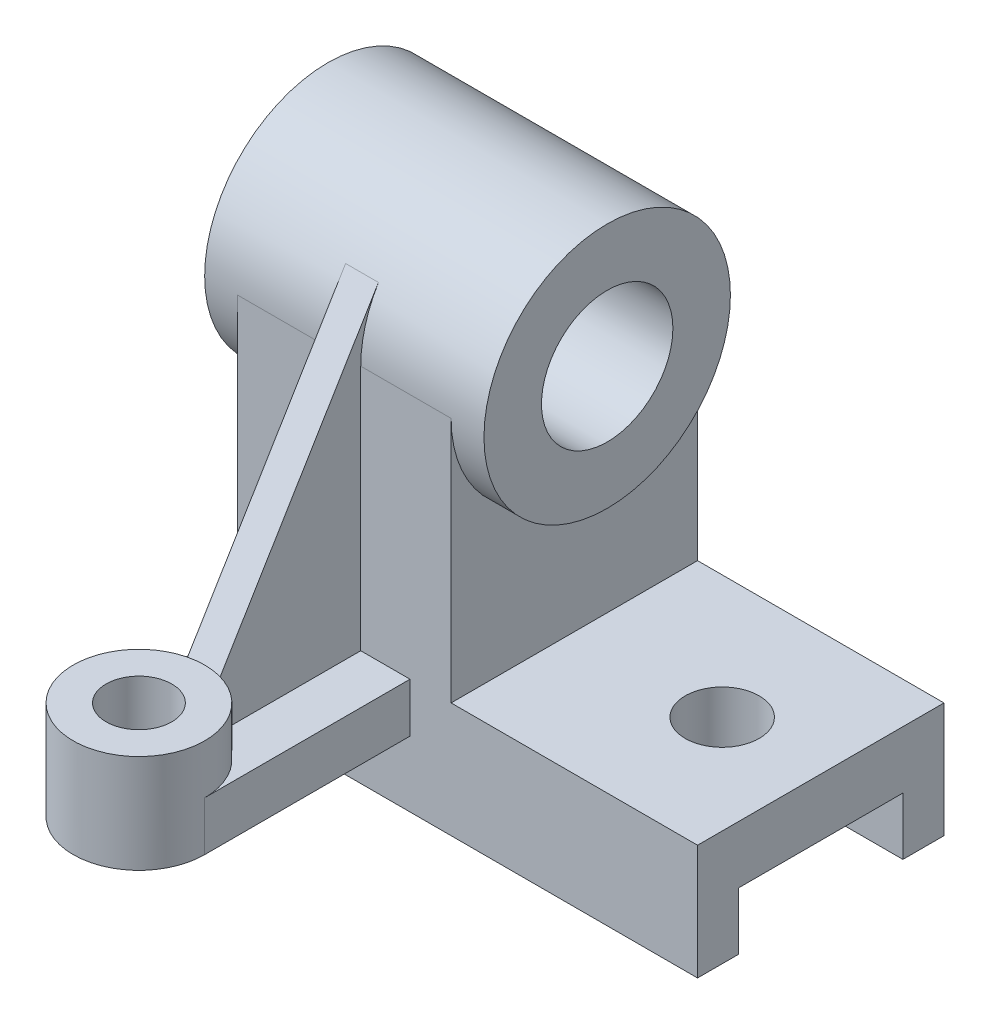
ISO-10303-21;
HEADER;
FILE_DESCRIPTION(('STEP AP214'),'2;1');
FILE_NAME('part.step','',(''),(''),'','','');
FILE_SCHEMA(('AUTOMOTIVE_DESIGN { 1 0 10303 214 1 1 1 1 }'));
ENDSEC;
DATA;
#1=APPLICATION_CONTEXT('core data for automotive mechanical design processes');
#2=APPLICATION_PROTOCOL_DEFINITION('international standard','automotive_design',2000,#1);
#3=PRODUCT_CONTEXT('',#1,'mechanical');
#4=PRODUCT('Part','Part','',(#3));
#5=PRODUCT_RELATED_PRODUCT_CATEGORY('part','',(#4));
#6=PRODUCT_DEFINITION_FORMATION('','',#4);
#7=PRODUCT_DEFINITION_CONTEXT('part definition',#1,'design');
#8=PRODUCT_DEFINITION('design','',#6,#7);
#9=PRODUCT_DEFINITION_SHAPE('','',#8);
#10=(LENGTH_UNIT() NAMED_UNIT(*) SI_UNIT(.MILLI.,.METRE.));
#11=(NAMED_UNIT(*) PLANE_ANGLE_UNIT() SI_UNIT($,.RADIAN.));
#12=(NAMED_UNIT(*) SI_UNIT($,.STERADIAN.) SOLID_ANGLE_UNIT());
#13=UNCERTAINTY_MEASURE_WITH_UNIT(LENGTH_MEASURE(1.E-05),#10,'distance_accuracy_value','');
#14=(GEOMETRIC_REPRESENTATION_CONTEXT(3) GLOBAL_UNCERTAINTY_ASSIGNED_CONTEXT((#13)) GLOBAL_UNIT_ASSIGNED_CONTEXT((#10,
#11,#12)) REPRESENTATION_CONTEXT('',''));
#15=CARTESIAN_POINT('',(0.,0.,0.));
#16=DIRECTION('',(0.,0.,1.));
#17=DIRECTION('',(1.,0.,0.));
#18=AXIS2_PLACEMENT_3D('',#15,#16,#17);
#19=CARTESIAN_POINT('',(0.,-60.,0.));
#20=DIRECTION('',(0.,1.,0.));
#21=DIRECTION('',(0.,0.,1.));
#22=AXIS2_PLACEMENT_3D('',#19,#20,#21);
#23=PLANE('',#22);
#24=CARTESIAN_POINT('',(0.,-60.,80.));
#25=DIRECTION('',(0.,1.,0.));
#26=DIRECTION('',(0.,0.,1.));
#27=AXIS2_PLACEMENT_3D('',#24,#25,#26);
#28=CIRCLE('',#27,16.);
#29=CARTESIAN_POINT('',(-4.,-60.,64.5080666151703));
#30=VERTEX_POINT('',#29);
#31=CARTESIAN_POINT('',(-16.,-60.,80.));
#32=VERTEX_POINT('',#31);
#33=EDGE_CURVE('E195',#30,#32,#28,.T.);
#34=ORIENTED_EDGE('',*,*,#33,.F.);
#35=DIRECTION('',(0.,0.,-1.));
#36=VECTOR('',#35,1.);
#37=CARTESIAN_POINT('',(-4.,-60.,0.));
#38=LINE('',#37,#36);
#39=CARTESIAN_POINT('',(-4.,-60.,30.));
#40=VERTEX_POINT('',#39);
#41=EDGE_CURVE('E191',#30,#40,#38,.T.);
#42=ORIENTED_EDGE('',*,*,#41,.T.);
#43=DIRECTION('',(-1.,0.,0.));
#44=VECTOR('',#43,1.);
#45=CARTESIAN_POINT('',(-16.,-60.,30.));
#46=LINE('',#45,#44);
#47=CARTESIAN_POINT('',(-16.,-60.,30.));
#48=VERTEX_POINT('',#47);
#49=EDGE_CURVE('E172',#40,#48,#46,.T.);
#50=ORIENTED_EDGE('',*,*,#49,.T.);
#51=DIRECTION('',(0.,0.,1.));
#52=VECTOR('',#51,1.);
#53=CARTESIAN_POINT('',(-16.,-60.,30.));
#54=LINE('',#53,#52);
#55=EDGE_CURVE('E227',#48,#32,#54,.T.);
#56=ORIENTED_EDGE('',*,*,#55,.T.);
#57=EDGE_LOOP('',(#34,#42,#50,#56));
#58=FACE_BOUND('',#57,.T.);
#59=ADVANCED_FACE('F41',(#58),#23,.T.);
#60=DIRECTION('',(0.,0.,-1.));
#61=VECTOR('',#60,1.);
#62=CARTESIAN_POINT('',(4.,-60.,0.));
#63=LINE('',#62,#61);
#64=CARTESIAN_POINT('',(4.,-60.,64.5080666151703));
#65=VERTEX_POINT('',#64);
#66=CARTESIAN_POINT('',(4.,-60.,30.));
#67=VERTEX_POINT('',#66);
#68=EDGE_CURVE('E215',#65,#67,#63,.T.);
#69=ORIENTED_EDGE('',*,*,#68,.F.);
#70=CARTESIAN_POINT('',(16.,-60.,80.));
#71=VERTEX_POINT('',#70);
#72=EDGE_CURVE('E234',#71,#65,#28,.T.);
#73=ORIENTED_EDGE('',*,*,#72,.F.);
#74=DIRECTION('',(0.,0.,-1.));
#75=VECTOR('',#74,1.);
#76=CARTESIAN_POINT('',(16.,-60.,30.));
#77=LINE('',#76,#75);
#78=CARTESIAN_POINT('',(16.,-60.,30.));
#79=VERTEX_POINT('',#78);
#80=EDGE_CURVE('E186',#71,#79,#77,.T.);
#81=ORIENTED_EDGE('',*,*,#80,.T.);
#82=EDGE_CURVE('E190',#79,#67,#46,.T.);
#83=ORIENTED_EDGE('',*,*,#82,.T.);
#84=EDGE_LOOP('',(#69,#73,#81,#83));
#85=FACE_BOUND('',#84,.T.);
#86=ADVANCED_FACE('F410',(#85),#23,.T.);
#87=CARTESIAN_POINT('',(0.,-60.,80.));
#88=DIRECTION('',(0.,1.,0.));
#89=DIRECTION('',(0.,0.,1.));
#90=AXIS2_PLACEMENT_3D('',#87,#88,#89);
#91=CYLINDRICAL_SURFACE('',#90,16.);
#92=DIRECTION('',(0.,1.,0.));
#93=VECTOR('',#92,1.);
#94=CARTESIAN_POINT('',(4.,-60.,64.5080666151703));
#95=LINE('',#94,#93);
#96=CARTESIAN_POINT('',(4.,-48.8420392680333,64.5080666151703));
#97=VERTEX_POINT('',#96);
#98=EDGE_CURVE('E60',#97,#65,#95,.F.);
#99=ORIENTED_EDGE('',*,*,#98,.F.);
#100=CARTESIAN_POINT('',(0.,-74.5174445363139,80.));
#101=DIRECTION('',(0.,-0.516619848709566,-0.856214886532175));
#102=DIRECTION('',(0.,0.856214886532175,-0.516619848709566));
#103=AXIS2_PLACEMENT_3D('',#100,#101,#102);
#104=ELLIPSE('',#103,30.9705483441363,16.);
#105=CARTESIAN_POINT('',(0.,-48.,64.));
#106=VERTEX_POINT('',#105);
#107=EDGE_CURVE('E219',#106,#97,#104,.T.);
#108=ORIENTED_EDGE('',*,*,#107,.F.);
#109=CARTESIAN_POINT('',(0.,-48.,80.));
#110=DIRECTION('',(0.,1.,0.));
#111=DIRECTION('',(0.,0.,1.));
#112=AXIS2_PLACEMENT_3D('',#109,#110,#111);
#113=CIRCLE('',#112,16.);
#114=EDGE_CURVE('E230',#106,#106,#113,.T.);
#115=ORIENTED_EDGE('',*,*,#114,.F.);
#116=CARTESIAN_POINT('',(-4.,-48.8420392680333,64.5080666151703));
#117=VERTEX_POINT('',#116);
#118=EDGE_CURVE('E64',#117,#106,#104,.T.);
#119=ORIENTED_EDGE('',*,*,#118,.F.);
#120=DIRECTION('',(0.,1.,0.));
#121=VECTOR('',#120,1.);
#122=CARTESIAN_POINT('',(-4.,-60.,64.5080666151703));
#123=LINE('',#122,#121);
#124=EDGE_CURVE('E192',#117,#30,#123,.F.);
#125=ORIENTED_EDGE('',*,*,#124,.T.);
#126=ORIENTED_EDGE('',*,*,#33,.T.);
#127=DIRECTION('',(0.,1.,0.));
#128=VECTOR('',#127,1.);
#129=CARTESIAN_POINT('',(-16.,-72.,80.));
#130=LINE('',#129,#128);
#131=CARTESIAN_POINT('',(-16.,-72.,80.));
#132=VERTEX_POINT('',#131);
#133=EDGE_CURVE('E49',#132,#32,#130,.T.);
#134=ORIENTED_EDGE('',*,*,#133,.F.);
#135=CARTESIAN_POINT('',(0.,-72.,80.));
#136=DIRECTION('',(0.,1.,0.));
#137=DIRECTION('',(0.,0.,1.));
#138=AXIS2_PLACEMENT_3D('',#135,#136,#137);
#139=CIRCLE('',#138,16.);
#140=CARTESIAN_POINT('',(16.,-72.,80.));
#141=VERTEX_POINT('',#140);
#142=EDGE_CURVE('E11',#141,#132,#139,.F.);
#143=ORIENTED_EDGE('',*,*,#142,.F.);
#144=DIRECTION('',(0.,1.,0.));
#145=VECTOR('',#144,1.);
#146=CARTESIAN_POINT('',(16.,-72.,80.));
#147=LINE('',#146,#145);
#148=EDGE_CURVE('E333',#71,#141,#147,.F.);
#149=ORIENTED_EDGE('',*,*,#148,.F.);
#150=ORIENTED_EDGE('',*,*,#72,.T.);
#151=EDGE_LOOP('',(#99,#108,#115,#119,#125,#126,#134,#143,#149,#150));
#152=FACE_BOUND('',#151,.T.);
#153=ADVANCED_FACE('F42',(#152),#91,.T.);
#154=CARTESIAN_POINT('',(86.,-88.,30.));
#155=DIRECTION('',(0.,1.,0.));
#156=DIRECTION('',(-1.,0.,0.));
#157=AXIS2_PLACEMENT_3D('',#154,#155,#156);
#158=PLANE('',#157);
#159=DIRECTION('',(0.,0.,-1.));
#160=VECTOR('',#159,1.);
#161=CARTESIAN_POINT('',(86.,-88.,30.));
#162=LINE('',#161,#160);
#163=CARTESIAN_POINT('',(86.,-88.,-20.));
#164=VERTEX_POINT('',#163);
#165=CARTESIAN_POINT('',(86.,-88.,-30.));
#166=VERTEX_POINT('',#165);
#167=EDGE_CURVE('E303',#164,#166,#162,.T.);
#168=ORIENTED_EDGE('',*,*,#167,.F.);
#169=DIRECTION('',(1.,0.,0.));
#170=VECTOR('',#169,1.);
#171=CARTESIAN_POINT('',(-34.,-88.,-20.));
#172=LINE('',#171,#170);
#173=CARTESIAN_POINT('',(-26.,-88.,-20.));
#174=VERTEX_POINT('',#173);
#175=EDGE_CURVE('E266',#174,#164,#172,.T.);
#176=ORIENTED_EDGE('',*,*,#175,.F.);
#177=DIRECTION('',(0.,0.,-1.));
#178=VECTOR('',#177,1.);
#179=CARTESIAN_POINT('',(-26.,-88.,30.));
#180=LINE('',#179,#178);
#181=CARTESIAN_POINT('',(-26.,-88.,-30.));
#182=VERTEX_POINT('',#181);
#183=EDGE_CURVE('E306',#174,#182,#180,.T.);
#184=ORIENTED_EDGE('',*,*,#183,.T.);
#185=DIRECTION('',(1.,0.,0.));
#186=VECTOR('',#185,1.);
#187=CARTESIAN_POINT('',(86.,-88.,-30.));
#188=LINE('',#187,#186);
#189=EDGE_CURVE('E292',#182,#166,#188,.T.);
#190=ORIENTED_EDGE('',*,*,#189,.T.);
#191=EDGE_LOOP('',(#168,#176,#184,#190));
#192=FACE_BOUND('',#191,.T.);
#193=ADVANCED_FACE('F401',(#192),#158,.F.);
#194=CARTESIAN_POINT('',(86.,-60.,30.));
#195=DIRECTION('',(-1.,0.,0.));
#196=DIRECTION('',(0.,0.,1.));
#197=AXIS2_PLACEMENT_3D('',#194,#195,#196);
#198=PLANE('',#197);
#199=DIRECTION('',(0.,-1.,0.));
#200=VECTOR('',#199,1.);
#201=CARTESIAN_POINT('',(86.,-88.,20.));
#202=LINE('',#201,#200);
#203=CARTESIAN_POINT('',(86.,-74.,20.));
#204=VERTEX_POINT('',#203);
#205=CARTESIAN_POINT('',(86.,-88.,20.));
#206=VERTEX_POINT('',#205);
#207=EDGE_CURVE('E253',#204,#206,#202,.T.);
#208=ORIENTED_EDGE('',*,*,#207,.F.);
#209=DIRECTION('',(0.,0.,1.));
#210=VECTOR('',#209,1.);
#211=CARTESIAN_POINT('',(86.,-74.,20.));
#212=LINE('',#211,#210);
#213=CARTESIAN_POINT('',(86.,-74.,-20.));
#214=VERTEX_POINT('',#213);
#215=EDGE_CURVE('E260',#214,#204,#212,.T.);
#216=ORIENTED_EDGE('',*,*,#215,.F.);
#217=DIRECTION('',(0.,1.,0.));
#218=VECTOR('',#217,1.);
#219=CARTESIAN_POINT('',(86.,-88.,-20.));
#220=LINE('',#219,#218);
#221=EDGE_CURVE('E255',#164,#214,#220,.T.);
#222=ORIENTED_EDGE('',*,*,#221,.F.);
#223=ORIENTED_EDGE('',*,*,#167,.T.);
#224=DIRECTION('',(0.,1.,0.));
#225=VECTOR('',#224,1.);
#226=CARTESIAN_POINT('',(86.,-60.,-30.));
#227=LINE('',#226,#225);
#228=CARTESIAN_POINT('',(86.,-60.,-30.));
#229=VERTEX_POINT('',#228);
#230=EDGE_CURVE('E291',#166,#229,#227,.T.);
#231=ORIENTED_EDGE('',*,*,#230,.T.);
#232=DIRECTION('',(0.,0.,-1.));
#233=VECTOR('',#232,1.);
#234=CARTESIAN_POINT('',(86.,-60.,30.));
#235=LINE('',#234,#233);
#236=CARTESIAN_POINT('',(86.,-60.,30.));
#237=VERTEX_POINT('',#236);
#238=EDGE_CURVE('E304',#237,#229,#235,.T.);
#239=ORIENTED_EDGE('',*,*,#238,.F.);
#240=DIRECTION('',(0.,1.,0.));
#241=VECTOR('',#240,1.);
#242=CARTESIAN_POINT('',(86.,-60.,30.));
#243=LINE('',#242,#241);
#244=CARTESIAN_POINT('',(86.,-88.,30.));
#245=VERTEX_POINT('',#244);
#246=EDGE_CURVE('E276',#245,#237,#243,.T.);
#247=ORIENTED_EDGE('',*,*,#246,.F.);
#248=EDGE_CURVE('E302',#245,#206,#162,.T.);
#249=ORIENTED_EDGE('',*,*,#248,.T.);
#250=EDGE_LOOP('',(#208,#216,#222,#223,#231,#239,#247,#249));
#251=FACE_BOUND('',#250,.T.);
#252=ADVANCED_FACE('F390',(#251),#198,.F.);
#253=CARTESIAN_POINT('',(34.,0.,0.));
#254=DIRECTION('',(-1.,0.,0.));
#255=DIRECTION('',(0.,0.,1.));
#256=AXIS2_PLACEMENT_3D('',#253,#254,#255);
#257=CYLINDRICAL_SURFACE('',#256,30.);
#258=CARTESIAN_POINT('',(34.,0.,0.));
#259=DIRECTION('',(1.,0.,0.));
#260=DIRECTION('',(0.,0.,-1.));
#261=AXIS2_PLACEMENT_3D('',#258,#259,#260);
#262=CIRCLE('',#261,30.);
#263=CARTESIAN_POINT('',(34.,0.,-30.));
#264=VERTEX_POINT('',#263);
#265=EDGE_CURVE('E322',#264,#264,#262,.T.);
#266=ORIENTED_EDGE('',*,*,#265,.F.);
#267=EDGE_LOOP('',(#266));
#268=FACE_BOUND('',#267,.T.);
#269=DIRECTION('',(-1.,0.,0.));
#270=VECTOR('',#269,1.);
#271=CARTESIAN_POINT('',(-26.,0.,-30.));
#272=LINE('',#271,#270);
#273=CARTESIAN_POINT('',(26.,0.,-30.));
#274=VERTEX_POINT('',#273);
#275=CARTESIAN_POINT('',(-26.,0.,-30.));
#276=VERTEX_POINT('',#275);
#277=EDGE_CURVE('E271',#274,#276,#272,.T.);
#278=ORIENTED_EDGE('',*,*,#277,.T.);
#279=CARTESIAN_POINT('',(-26.,0.,0.));
#280=DIRECTION('',(1.,0.,0.));
#281=DIRECTION('',(0.,1.,0.));
#282=AXIS2_PLACEMENT_3D('',#279,#280,#281);
#283=CIRCLE('',#282,30.);
#284=CARTESIAN_POINT('',(-26.,0.,30.));
#285=VERTEX_POINT('',#284);
#286=EDGE_CURVE('E314',#285,#276,#283,.T.);
#287=ORIENTED_EDGE('',*,*,#286,.F.);
#288=DIRECTION('',(-1.,0.,0.));
#289=VECTOR('',#288,1.);
#290=CARTESIAN_POINT('',(-26.,0.,30.));
#291=LINE('',#290,#289);
#292=CARTESIAN_POINT('',(-4.,0.,30.));
#293=VERTEX_POINT('',#292);
#294=EDGE_CURVE('E274',#293,#285,#291,.T.);
#295=ORIENTED_EDGE('',*,*,#294,.F.);
#296=CARTESIAN_POINT('',(-4.,0.,0.));
#297=DIRECTION('',(1.,0.,0.));
#298=DIRECTION('',(0.,0.,-1.));
#299=AXIS2_PLACEMENT_3D('',#296,#297,#298);
#300=CIRCLE('',#299,30.);
#301=CARTESIAN_POINT('',(-4.,15.498595461287,25.6864465959653));
#302=VERTEX_POINT('',#301);
#303=EDGE_CURVE('E199',#302,#293,#300,.T.);
#304=ORIENTED_EDGE('',*,*,#303,.F.);
#305=DIRECTION('',(-1.,0.,0.));
#306=VECTOR('',#305,1.);
#307=CARTESIAN_POINT('',(34.,15.498595461287,25.6864465959652));
#308=LINE('',#307,#306);
#309=CARTESIAN_POINT('',(4.,15.498595461287,25.6864465959653));
#310=VERTEX_POINT('',#309);
#311=EDGE_CURVE('E220',#302,#310,#308,.F.);
#312=ORIENTED_EDGE('',*,*,#311,.T.);
#313=CARTESIAN_POINT('',(4.,0.,0.));
#314=DIRECTION('',(1.,0.,0.));
#315=DIRECTION('',(0.,0.,-1.));
#316=AXIS2_PLACEMENT_3D('',#313,#314,#315);
#317=CIRCLE('',#316,30.);
#318=CARTESIAN_POINT('',(4.,0.,30.));
#319=VERTEX_POINT('',#318);
#320=EDGE_CURVE('E207',#310,#319,#317,.T.);
#321=ORIENTED_EDGE('',*,*,#320,.T.);
#322=CARTESIAN_POINT('',(26.,0.,30.));
#323=VERTEX_POINT('',#322);
#324=EDGE_CURVE('E275',#323,#319,#291,.T.);
#325=ORIENTED_EDGE('',*,*,#324,.F.);
#326=CARTESIAN_POINT('',(26.,0.,0.));
#327=DIRECTION('',(-1.,0.,0.));
#328=DIRECTION('',(0.,-1.,0.));
#329=AXIS2_PLACEMENT_3D('',#326,#327,#328);
#330=CIRCLE('',#329,30.);
#331=EDGE_CURVE('E315',#274,#323,#330,.T.);
#332=ORIENTED_EDGE('',*,*,#331,.F.);
#333=EDGE_LOOP('',(#278,#287,#295,#304,#312,#321,#325,#332));
#334=FACE_BOUND('',#333,.T.);
#335=CARTESIAN_POINT('',(-34.,0.,0.));
#336=DIRECTION('',(1.,0.,0.));
#337=DIRECTION('',(0.,0.,-1.));
#338=AXIS2_PLACEMENT_3D('',#335,#336,#337);
#339=CIRCLE('',#338,30.);
#340=CARTESIAN_POINT('',(-34.,0.,-30.));
#341=VERTEX_POINT('',#340);
#342=EDGE_CURVE('E321',#341,#341,#339,.T.);
#343=ORIENTED_EDGE('',*,*,#342,.T.);
#344=EDGE_LOOP('',(#343));
#345=FACE_BOUND('',#344,.T.);
#346=ADVANCED_FACE('F356',(#268,#334,#345),#257,.T.);
#347=CARTESIAN_POINT('',(34.,0.,0.));
#348=DIRECTION('',(-1.,0.,0.));
#349=DIRECTION('',(0.,0.,1.));
#350=AXIS2_PLACEMENT_3D('',#347,#348,#349);
#351=CYLINDRICAL_SURFACE('',#350,16.);
#352=CARTESIAN_POINT('',(34.,0.,0.));
#353=DIRECTION('',(1.,0.,0.));
#354=DIRECTION('',(0.,0.,-1.));
#355=AXIS2_PLACEMENT_3D('',#352,#353,#354);
#356=CIRCLE('',#355,16.);
#357=CARTESIAN_POINT('',(34.,0.,-16.));
#358=VERTEX_POINT('',#357);
#359=EDGE_CURVE('E318',#358,#358,#356,.T.);
#360=ORIENTED_EDGE('',*,*,#359,.T.);
#361=EDGE_LOOP('',(#360));
#362=FACE_BOUND('',#361,.T.);
#363=CARTESIAN_POINT('',(-34.,0.,0.));
#364=DIRECTION('',(1.,0.,0.));
#365=DIRECTION('',(0.,0.,-1.));
#366=AXIS2_PLACEMENT_3D('',#363,#364,#365);
#367=CIRCLE('',#366,16.);
#368=CARTESIAN_POINT('',(-34.,0.,-16.));
#369=VERTEX_POINT('',#368);
#370=EDGE_CURVE('E320',#369,#369,#367,.T.);
#371=ORIENTED_EDGE('',*,*,#370,.F.);
#372=EDGE_LOOP('',(#371));
#373=FACE_BOUND('',#372,.T.);
#374=ADVANCED_FACE('F599',(#362,#373),#351,.F.);
#375=CARTESIAN_POINT('',(34.,0.,0.));
#376=DIRECTION('',(1.,0.,0.));
#377=DIRECTION('',(0.,0.,-1.));
#378=AXIS2_PLACEMENT_3D('',#375,#376,#377);
#379=PLANE('',#378);
#380=ORIENTED_EDGE('',*,*,#265,.T.);
#381=EDGE_LOOP('',(#380));
#382=FACE_BOUND('',#381,.T.);
#383=ORIENTED_EDGE('',*,*,#359,.F.);
#384=EDGE_LOOP('',(#383));
#385=FACE_BOUND('',#384,.T.);
#386=ADVANCED_FACE('F606',(#382,#385),#379,.T.);
#387=CARTESIAN_POINT('',(-34.,0.,0.));
#388=DIRECTION('',(1.,0.,0.));
#389=DIRECTION('',(0.,0.,-1.));
#390=AXIS2_PLACEMENT_3D('',#387,#388,#389);
#391=PLANE('',#390);
#392=ORIENTED_EDGE('',*,*,#342,.F.);
#393=EDGE_LOOP('',(#392));
#394=FACE_BOUND('',#393,.T.);
#395=ORIENTED_EDGE('',*,*,#370,.T.);
#396=EDGE_LOOP('',(#395));
#397=FACE_BOUND('',#396,.T.);
#398=ADVANCED_FACE('F593',(#394,#397),#391,.F.);
#399=CARTESIAN_POINT('',(-26.,-88.,30.));
#400=DIRECTION('',(1.,0.,0.));
#401=DIRECTION('',(0.,1.,0.));
#402=AXIS2_PLACEMENT_3D('',#399,#400,#401);
#403=PLANE('',#402);
#404=DIRECTION('',(0.,0.,1.));
#405=VECTOR('',#404,1.);
#406=CARTESIAN_POINT('',(-26.,-74.,30.));
#407=LINE('',#406,#405);
#408=CARTESIAN_POINT('',(-26.,-74.,-20.));
#409=VERTEX_POINT('',#408);
#410=CARTESIAN_POINT('',(-26.,-74.,20.));
#411=VERTEX_POINT('',#410);
#412=EDGE_CURVE('E263',#409,#411,#407,.T.);
#413=ORIENTED_EDGE('',*,*,#412,.T.);
#414=DIRECTION('',(0.,-1.,0.));
#415=VECTOR('',#414,1.);
#416=CARTESIAN_POINT('',(-26.,-88.,20.));
#417=LINE('',#416,#415);
#418=CARTESIAN_POINT('',(-26.,-88.,20.));
#419=VERTEX_POINT('',#418);
#420=EDGE_CURVE('E335',#411,#419,#417,.T.);
#421=ORIENTED_EDGE('',*,*,#420,.T.);
#422=CARTESIAN_POINT('',(-26.,-88.,30.));
#423=VERTEX_POINT('',#422);
#424=EDGE_CURVE('E310',#423,#419,#180,.T.);
#425=ORIENTED_EDGE('',*,*,#424,.F.);
#426=DIRECTION('',(0.,-1.,0.));
#427=VECTOR('',#426,1.);
#428=CARTESIAN_POINT('',(-26.,-88.,30.));
#429=LINE('',#428,#427);
#430=EDGE_CURVE('E273',#285,#423,#429,.T.);
#431=ORIENTED_EDGE('',*,*,#430,.F.);
#432=ORIENTED_EDGE('',*,*,#286,.T.);
#433=DIRECTION('',(0.,-1.,0.));
#434=VECTOR('',#433,1.);
#435=CARTESIAN_POINT('',(-26.,-88.,-30.));
#436=LINE('',#435,#434);
#437=EDGE_CURVE('E290',#276,#182,#436,.T.);
#438=ORIENTED_EDGE('',*,*,#437,.T.);
#439=ORIENTED_EDGE('',*,*,#183,.F.);
#440=DIRECTION('',(0.,1.,0.));
#441=VECTOR('',#440,1.);
#442=CARTESIAN_POINT('',(-26.,-88.,-20.));
#443=LINE('',#442,#441);
#444=EDGE_CURVE('E330',#174,#409,#443,.T.);
#445=ORIENTED_EDGE('',*,*,#444,.T.);
#446=EDGE_LOOP('',(#413,#421,#425,#431,#432,#438,#439,#445));
#447=FACE_BOUND('',#446,.T.);
#448=ADVANCED_FACE('F380',(#447),#403,.F.);
#449=ORIENTED_EDGE('',*,*,#248,.F.);
#450=DIRECTION('',(1.,0.,0.));
#451=VECTOR('',#450,1.);
#452=CARTESIAN_POINT('',(86.,-88.,30.));
#453=LINE('',#452,#451);
#454=EDGE_CURVE('E280',#423,#245,#453,.T.);
#455=ORIENTED_EDGE('',*,*,#454,.F.);
#456=ORIENTED_EDGE('',*,*,#424,.T.);
#457=DIRECTION('',(1.,0.,0.));
#458=VECTOR('',#457,1.);
#459=CARTESIAN_POINT('',(-34.,-88.,20.));
#460=LINE('',#459,#458);
#461=EDGE_CURVE('E257',#419,#206,#460,.T.);
#462=ORIENTED_EDGE('',*,*,#461,.T.);
#463=EDGE_LOOP('',(#449,#455,#456,#462));
#464=FACE_BOUND('',#463,.T.);
#465=ADVANCED_FACE('F383',(#464),#158,.F.);
#466=CARTESIAN_POINT('',(26.,-60.,30.));
#467=DIRECTION('',(0.,-1.,0.));
#468=DIRECTION('',(0.,0.,-1.));
#469=AXIS2_PLACEMENT_3D('',#466,#467,#468);
#470=PLANE('',#469);
#471=CARTESIAN_POINT('',(62.,-60.,0.));
#472=DIRECTION('',(0.,1.,0.));
#473=DIRECTION('',(0.,0.,1.));
#474=AXIS2_PLACEMENT_3D('',#471,#472,#473);
#475=CIRCLE('',#474,9.);
#476=CARTESIAN_POINT('',(62.,-60.,9.));
#477=VERTEX_POINT('',#476);
#478=EDGE_CURVE('E242',#477,#477,#475,.T.);
#479=ORIENTED_EDGE('',*,*,#478,.F.);
#480=EDGE_LOOP('',(#479));
#481=FACE_BOUND('',#480,.T.);
#482=DIRECTION('',(-1.,0.,0.));
#483=VECTOR('',#482,1.);
#484=CARTESIAN_POINT('',(26.,-60.,-30.));
#485=LINE('',#484,#483);
#486=CARTESIAN_POINT('',(26.,-60.,-30.));
#487=VERTEX_POINT('',#486);
#488=EDGE_CURVE('E293',#229,#487,#485,.T.);
#489=ORIENTED_EDGE('',*,*,#488,.T.);
#490=DIRECTION('',(0.,0.,-1.));
#491=VECTOR('',#490,1.);
#492=CARTESIAN_POINT('',(26.,-60.,30.));
#493=LINE('',#492,#491);
#494=CARTESIAN_POINT('',(26.,-60.,30.));
#495=VERTEX_POINT('',#494);
#496=EDGE_CURVE('E289',#495,#487,#493,.T.);
#497=ORIENTED_EDGE('',*,*,#496,.F.);
#498=DIRECTION('',(-1.,0.,0.));
#499=VECTOR('',#498,1.);
#500=CARTESIAN_POINT('',(26.,-60.,30.));
#501=LINE('',#500,#499);
#502=EDGE_CURVE('E283',#237,#495,#501,.T.);
#503=ORIENTED_EDGE('',*,*,#502,.F.);
#504=ORIENTED_EDGE('',*,*,#238,.T.);
#505=EDGE_LOOP('',(#489,#497,#503,#504));
#506=FACE_BOUND('',#505,.T.);
#507=ADVANCED_FACE('F393',(#481,#506),#470,.F.);
#508=CARTESIAN_POINT('',(26.,0.,30.));
#509=DIRECTION('',(-1.,0.,0.));
#510=DIRECTION('',(0.,-1.,0.));
#511=AXIS2_PLACEMENT_3D('',#508,#509,#510);
#512=PLANE('',#511);
#513=DIRECTION('',(0.,1.,0.));
#514=VECTOR('',#513,1.);
#515=CARTESIAN_POINT('',(26.,0.,-30.));
#516=LINE('',#515,#514);
#517=EDGE_CURVE('E300',#487,#274,#516,.T.);
#518=ORIENTED_EDGE('',*,*,#517,.T.);
#519=ORIENTED_EDGE('',*,*,#331,.T.);
#520=DIRECTION('',(0.,1.,0.));
#521=VECTOR('',#520,1.);
#522=CARTESIAN_POINT('',(26.,0.,30.));
#523=LINE('',#522,#521);
#524=EDGE_CURVE('E281',#495,#323,#523,.T.);
#525=ORIENTED_EDGE('',*,*,#524,.F.);
#526=ORIENTED_EDGE('',*,*,#496,.T.);
#527=EDGE_LOOP('',(#518,#519,#525,#526));
#528=FACE_BOUND('',#527,.T.);
#529=ADVANCED_FACE('F364',(#528),#512,.F.);
#530=CARTESIAN_POINT('',(0.,0.,30.));
#531=DIRECTION('',(0.,0.,-1.));
#532=DIRECTION('',(-1.,0.,0.));
#533=AXIS2_PLACEMENT_3D('',#530,#531,#532);
#534=PLANE('',#533);
#535=ORIENTED_EDGE('',*,*,#324,.T.);
#536=DIRECTION('',(0.,-1.,0.));
#537=VECTOR('',#536,1.);
#538=CARTESIAN_POINT('',(4.,0.,30.));
#539=LINE('',#538,#537);
#540=EDGE_CURVE('E209',#319,#67,#539,.T.);
#541=ORIENTED_EDGE('',*,*,#540,.T.);
#542=ORIENTED_EDGE('',*,*,#82,.F.);
#543=DIRECTION('',(0.,1.,0.));
#544=VECTOR('',#543,1.);
#545=CARTESIAN_POINT('',(16.,-72.,30.));
#546=LINE('',#545,#544);
#547=CARTESIAN_POINT('',(16.,-72.,30.));
#548=VERTEX_POINT('',#547);
#549=EDGE_CURVE('E238',#548,#79,#546,.T.);
#550=ORIENTED_EDGE('',*,*,#549,.F.);
#551=DIRECTION('',(-1.,0.,0.));
#552=VECTOR('',#551,1.);
#553=CARTESIAN_POINT('',(-16.,-72.,30.));
#554=LINE('',#553,#552);
#555=CARTESIAN_POINT('',(-16.,-72.,30.));
#556=VERTEX_POINT('',#555);
#557=EDGE_CURVE('E236',#548,#556,#554,.T.);
#558=ORIENTED_EDGE('',*,*,#557,.T.);
#559=DIRECTION('',(0.,1.,0.));
#560=VECTOR('',#559,1.);
#561=CARTESIAN_POINT('',(-16.,-72.,30.));
#562=LINE('',#561,#560);
#563=EDGE_CURVE('E181',#556,#48,#562,.T.);
#564=ORIENTED_EDGE('',*,*,#563,.T.);
#565=ORIENTED_EDGE('',*,*,#49,.F.);
#566=DIRECTION('',(0.,-1.,0.));
#567=VECTOR('',#566,1.);
#568=CARTESIAN_POINT('',(-4.,0.,30.));
#569=LINE('',#568,#567);
#570=EDGE_CURVE('E177',#293,#40,#569,.T.);
#571=ORIENTED_EDGE('',*,*,#570,.F.);
#572=ORIENTED_EDGE('',*,*,#294,.T.);
#573=ORIENTED_EDGE('',*,*,#430,.T.);
#574=ORIENTED_EDGE('',*,*,#454,.T.);
#575=ORIENTED_EDGE('',*,*,#246,.T.);
#576=ORIENTED_EDGE('',*,*,#502,.T.);
#577=ORIENTED_EDGE('',*,*,#524,.T.);
#578=EDGE_LOOP('',(#535,#541,#542,#550,#558,#564,#565,#571,#572,#573,#574,#575,#576,#577));
#579=FACE_BOUND('',#578,.T.);
#580=ADVANCED_FACE('F180',(#579),#534,.F.);
#581=CARTESIAN_POINT('',(0.,0.,-30.));
#582=DIRECTION('',(0.,0.,-1.));
#583=DIRECTION('',(-1.,0.,0.));
#584=AXIS2_PLACEMENT_3D('',#581,#582,#583);
#585=PLANE('',#584);
#586=ORIENTED_EDGE('',*,*,#230,.F.);
#587=ORIENTED_EDGE('',*,*,#189,.F.);
#588=ORIENTED_EDGE('',*,*,#437,.F.);
#589=ORIENTED_EDGE('',*,*,#277,.F.);
#590=ORIENTED_EDGE('',*,*,#517,.F.);
#591=ORIENTED_EDGE('',*,*,#488,.F.);
#592=EDGE_LOOP('',(#586,#587,#588,#589,#590,#591));
#593=FACE_BOUND('',#592,.T.);
#594=ADVANCED_FACE('F373',(#593),#585,.T.);
#595=CARTESIAN_POINT('',(-34.,-88.,20.));
#596=DIRECTION('',(0.,0.,1.));
#597=DIRECTION('',(1.,0.,0.));
#598=AXIS2_PLACEMENT_3D('',#595,#596,#597);
#599=PLANE('',#598);
#600=ORIENTED_EDGE('',*,*,#207,.T.);
#601=ORIENTED_EDGE('',*,*,#461,.F.);
#602=ORIENTED_EDGE('',*,*,#420,.F.);
#603=DIRECTION('',(1.,0.,0.));
#604=VECTOR('',#603,1.);
#605=CARTESIAN_POINT('',(-34.,-74.,20.));
#606=LINE('',#605,#604);
#607=EDGE_CURVE('E261',#411,#204,#606,.T.);
#608=ORIENTED_EDGE('',*,*,#607,.T.);
#609=EDGE_LOOP('',(#600,#601,#602,#608));
#610=FACE_BOUND('',#609,.T.);
#611=ADVANCED_FACE('F433',(#610),#599,.F.);
#612=CARTESIAN_POINT('',(-34.,-88.,-20.));
#613=DIRECTION('',(0.,0.,-1.));
#614=DIRECTION('',(-1.,0.,0.));
#615=AXIS2_PLACEMENT_3D('',#612,#613,#614);
#616=PLANE('',#615);
#617=ORIENTED_EDGE('',*,*,#221,.T.);
#618=DIRECTION('',(1.,0.,0.));
#619=VECTOR('',#618,1.);
#620=CARTESIAN_POINT('',(-34.,-74.,-20.));
#621=LINE('',#620,#619);
#622=EDGE_CURVE('E262',#409,#214,#621,.T.);
#623=ORIENTED_EDGE('',*,*,#622,.F.);
#624=ORIENTED_EDGE('',*,*,#444,.F.);
#625=ORIENTED_EDGE('',*,*,#175,.T.);
#626=EDGE_LOOP('',(#617,#623,#624,#625));
#627=FACE_BOUND('',#626,.T.);
#628=ADVANCED_FACE('F427',(#627),#616,.F.);
#629=CARTESIAN_POINT('',(-34.,-74.,20.));
#630=DIRECTION('',(0.,1.,0.));
#631=DIRECTION('',(0.,0.,1.));
#632=AXIS2_PLACEMENT_3D('',#629,#630,#631);
#633=PLANE('',#632);
#634=CARTESIAN_POINT('',(62.,-74.,0.));
#635=DIRECTION('',(0.,1.,0.));
#636=DIRECTION('',(0.,0.,1.));
#637=AXIS2_PLACEMENT_3D('',#634,#635,#636);
#638=CIRCLE('',#637,9.);
#639=CARTESIAN_POINT('',(62.,-74.,9.));
#640=VERTEX_POINT('',#639);
#641=EDGE_CURVE('E247',#640,#640,#638,.T.);
#642=ORIENTED_EDGE('',*,*,#641,.T.);
#643=EDGE_LOOP('',(#642));
#644=FACE_BOUND('',#643,.T.);
#645=ORIENTED_EDGE('',*,*,#215,.T.);
#646=ORIENTED_EDGE('',*,*,#607,.F.);
#647=ORIENTED_EDGE('',*,*,#412,.F.);
#648=ORIENTED_EDGE('',*,*,#622,.T.);
#649=EDGE_LOOP('',(#645,#646,#647,#648));
#650=FACE_BOUND('',#649,.T.);
#651=ADVANCED_FACE('F422',(#644,#650),#633,.F.);
#652=CARTESIAN_POINT('',(62.,-88.,0.));
#653=DIRECTION('',(0.,1.,0.));
#654=DIRECTION('',(0.,0.,1.));
#655=AXIS2_PLACEMENT_3D('',#652,#653,#654);
#656=CYLINDRICAL_SURFACE('',#655,9.);
#657=ORIENTED_EDGE('',*,*,#478,.T.);
#658=EDGE_LOOP('',(#657));
#659=FACE_BOUND('',#658,.T.);
#660=ORIENTED_EDGE('',*,*,#641,.F.);
#661=EDGE_LOOP('',(#660));
#662=FACE_BOUND('',#661,.T.);
#663=ADVANCED_FACE('F421',(#659,#662),#656,.F.);
#664=CARTESIAN_POINT('',(-16.,-72.,30.));
#665=DIRECTION('',(-1.,0.,0.));
#666=DIRECTION('',(0.,0.,1.));
#667=AXIS2_PLACEMENT_3D('',#664,#665,#666);
#668=PLANE('',#667);
#669=DIRECTION('',(0.,0.,1.));
#670=VECTOR('',#669,1.);
#671=CARTESIAN_POINT('',(-16.,-72.,30.));
#672=LINE('',#671,#670);
#673=EDGE_CURVE('E235',#556,#132,#672,.T.);
#674=ORIENTED_EDGE('',*,*,#673,.T.);
#675=ORIENTED_EDGE('',*,*,#133,.T.);
#676=ORIENTED_EDGE('',*,*,#55,.F.);
#677=ORIENTED_EDGE('',*,*,#563,.F.);
#678=EDGE_LOOP('',(#674,#675,#676,#677));
#679=FACE_BOUND('',#678,.T.);
#680=ADVANCED_FACE('F341',(#679),#668,.T.);
#681=CARTESIAN_POINT('',(16.,-72.,30.));
#682=DIRECTION('',(1.,0.,0.));
#683=DIRECTION('',(0.,0.,-1.));
#684=AXIS2_PLACEMENT_3D('',#681,#682,#683);
#685=PLANE('',#684);
#686=ORIENTED_EDGE('',*,*,#80,.F.);
#687=ORIENTED_EDGE('',*,*,#148,.T.);
#688=DIRECTION('',(0.,0.,-1.));
#689=VECTOR('',#688,1.);
#690=CARTESIAN_POINT('',(16.,-72.,30.));
#691=LINE('',#690,#689);
#692=EDGE_CURVE('E237',#141,#548,#691,.T.);
#693=ORIENTED_EDGE('',*,*,#692,.T.);
#694=ORIENTED_EDGE('',*,*,#549,.T.);
#695=EDGE_LOOP('',(#686,#687,#693,#694));
#696=FACE_BOUND('',#695,.T.);
#697=ADVANCED_FACE('F416',(#696),#685,.T.);
#698=CARTESIAN_POINT('',(0.,-72.,0.));
#699=DIRECTION('',(0.,1.,0.));
#700=DIRECTION('',(0.,0.,1.));
#701=AXIS2_PLACEMENT_3D('',#698,#699,#700);
#702=PLANE('',#701);
#703=ORIENTED_EDGE('',*,*,#673,.F.);
#704=ORIENTED_EDGE('',*,*,#557,.F.);
#705=ORIENTED_EDGE('',*,*,#692,.F.);
#706=ORIENTED_EDGE('',*,*,#142,.T.);
#707=EDGE_LOOP('',(#703,#704,#705,#706));
#708=FACE_BOUND('',#707,.T.);
#709=CARTESIAN_POINT('',(0.,-72.,80.));
#710=DIRECTION('',(0.,1.,0.));
#711=DIRECTION('',(0.,0.,1.));
#712=AXIS2_PLACEMENT_3D('',#709,#710,#711);
#713=CIRCLE('',#712,8.);
#714=CARTESIAN_POINT('',(0.,-72.,88.));
#715=VERTEX_POINT('',#714);
#716=EDGE_CURVE('E222',#715,#715,#713,.F.);
#717=ORIENTED_EDGE('',*,*,#716,.F.);
#718=EDGE_LOOP('',(#717));
#719=FACE_BOUND('',#718,.T.);
#720=ADVANCED_FACE('F418',(#708,#719),#702,.F.);
#721=CARTESIAN_POINT('',(0.,-48.,80.));
#722=DIRECTION('',(0.,1.,0.));
#723=DIRECTION('',(0.,0.,1.));
#724=AXIS2_PLACEMENT_3D('',#721,#722,#723);
#725=PLANE('',#724);
#726=ORIENTED_EDGE('',*,*,#114,.T.);
#727=EDGE_LOOP('',(#726));
#728=FACE_BOUND('',#727,.T.);
#729=CARTESIAN_POINT('',(0.,-48.,80.));
#730=DIRECTION('',(0.,1.,0.));
#731=DIRECTION('',(0.,0.,1.));
#732=AXIS2_PLACEMENT_3D('',#729,#730,#731);
#733=CIRCLE('',#732,8.);
#734=CARTESIAN_POINT('',(0.,-48.,88.));
#735=VERTEX_POINT('',#734);
#736=EDGE_CURVE('E221',#735,#735,#733,.T.);
#737=ORIENTED_EDGE('',*,*,#736,.F.);
#738=EDGE_LOOP('',(#737));
#739=FACE_BOUND('',#738,.T.);
#740=ADVANCED_FACE('F467',(#728,#739),#725,.T.);
#741=CARTESIAN_POINT('',(0.,-48.,80.));
#742=DIRECTION('',(0.,-1.,0.));
#743=DIRECTION('',(0.,0.,-1.));
#744=AXIS2_PLACEMENT_3D('',#741,#742,#743);
#745=CYLINDRICAL_SURFACE('',#744,8.);
#746=ORIENTED_EDGE('',*,*,#716,.T.);
#747=EDGE_LOOP('',(#746));
#748=FACE_BOUND('',#747,.T.);
#749=ORIENTED_EDGE('',*,*,#736,.T.);
#750=EDGE_LOOP('',(#749));
#751=FACE_BOUND('',#750,.T.);
#752=ADVANCED_FACE('F477',(#748,#751),#745,.F.);
#753=CARTESIAN_POINT('',(0.,-48.,64.));
#754=DIRECTION('',(0.,-0.516619848709566,-0.856214886532175));
#755=DIRECTION('',(0.,0.856214886532175,-0.516619848709566));
#756=AXIS2_PLACEMENT_3D('',#753,#754,#755);
#757=PLANE('',#756);
#758=ORIENTED_EDGE('',*,*,#118,.T.);
#759=ORIENTED_EDGE('',*,*,#107,.T.);
#760=DIRECTION('',(0.,0.856214886532175,-0.516619848709566));
#761=VECTOR('',#760,1.);
#762=CARTESIAN_POINT('',(4.,-48.,64.));
#763=LINE('',#762,#761);
#764=EDGE_CURVE('E205',#97,#310,#763,.T.);
#765=ORIENTED_EDGE('',*,*,#764,.T.);
#766=ORIENTED_EDGE('',*,*,#311,.F.);
#767=DIRECTION('',(0.,0.856214886532175,-0.516619848709566));
#768=VECTOR('',#767,1.);
#769=CARTESIAN_POINT('',(-4.,-48.,64.));
#770=LINE('',#769,#768);
#771=EDGE_CURVE('E202',#117,#302,#770,.T.);
#772=ORIENTED_EDGE('',*,*,#771,.F.);
#773=EDGE_LOOP('',(#758,#759,#765,#766,#772));
#774=FACE_BOUND('',#773,.T.);
#775=ADVANCED_FACE('F346',(#774),#757,.F.);
#776=CARTESIAN_POINT('',(4.,-29.,33.));
#777=DIRECTION('',(1.,0.,0.));
#778=DIRECTION('',(0.,0.,-1.));
#779=AXIS2_PLACEMENT_3D('',#776,#777,#778);
#780=PLANE('',#779);
#781=ORIENTED_EDGE('',*,*,#764,.F.);
#782=ORIENTED_EDGE('',*,*,#98,.T.);
#783=ORIENTED_EDGE('',*,*,#68,.T.);
#784=ORIENTED_EDGE('',*,*,#540,.F.);
#785=ORIENTED_EDGE('',*,*,#320,.F.);
#786=EDGE_LOOP('',(#781,#782,#783,#784,#785));
#787=FACE_BOUND('',#786,.T.);
#788=ADVANCED_FACE('F351',(#787),#780,.T.);
#789=CARTESIAN_POINT('',(-4.,-29.,33.));
#790=DIRECTION('',(1.,0.,0.));
#791=DIRECTION('',(0.,0.,-1.));
#792=AXIS2_PLACEMENT_3D('',#789,#790,#791);
#793=PLANE('',#792);
#794=ORIENTED_EDGE('',*,*,#124,.F.);
#795=ORIENTED_EDGE('',*,*,#771,.T.);
#796=ORIENTED_EDGE('',*,*,#303,.T.);
#797=ORIENTED_EDGE('',*,*,#570,.T.);
#798=ORIENTED_EDGE('',*,*,#41,.F.);
#799=EDGE_LOOP('',(#794,#795,#796,#797,#798));
#800=FACE_BOUND('',#799,.T.);
#801=ADVANCED_FACE('F196',(#800),#793,.F.);
#802=CLOSED_SHELL('',(#59,#86,#153,#193,#252,#346,#374,#386,#398,#448,#465,#507,#529,#580,#594,
#611,#628,#651,#663,#680,#697,#720,#740,#752,#775,#788,#801));
#803=MANIFOLD_SOLID_BREP('B2',#802);
#804=ADVANCED_BREP_SHAPE_REPRESENTATION('',(#18,#803),#14);
#805=SHAPE_DEFINITION_REPRESENTATION(#9,#804);
ENDSEC;
END-ISO-10303-21;
